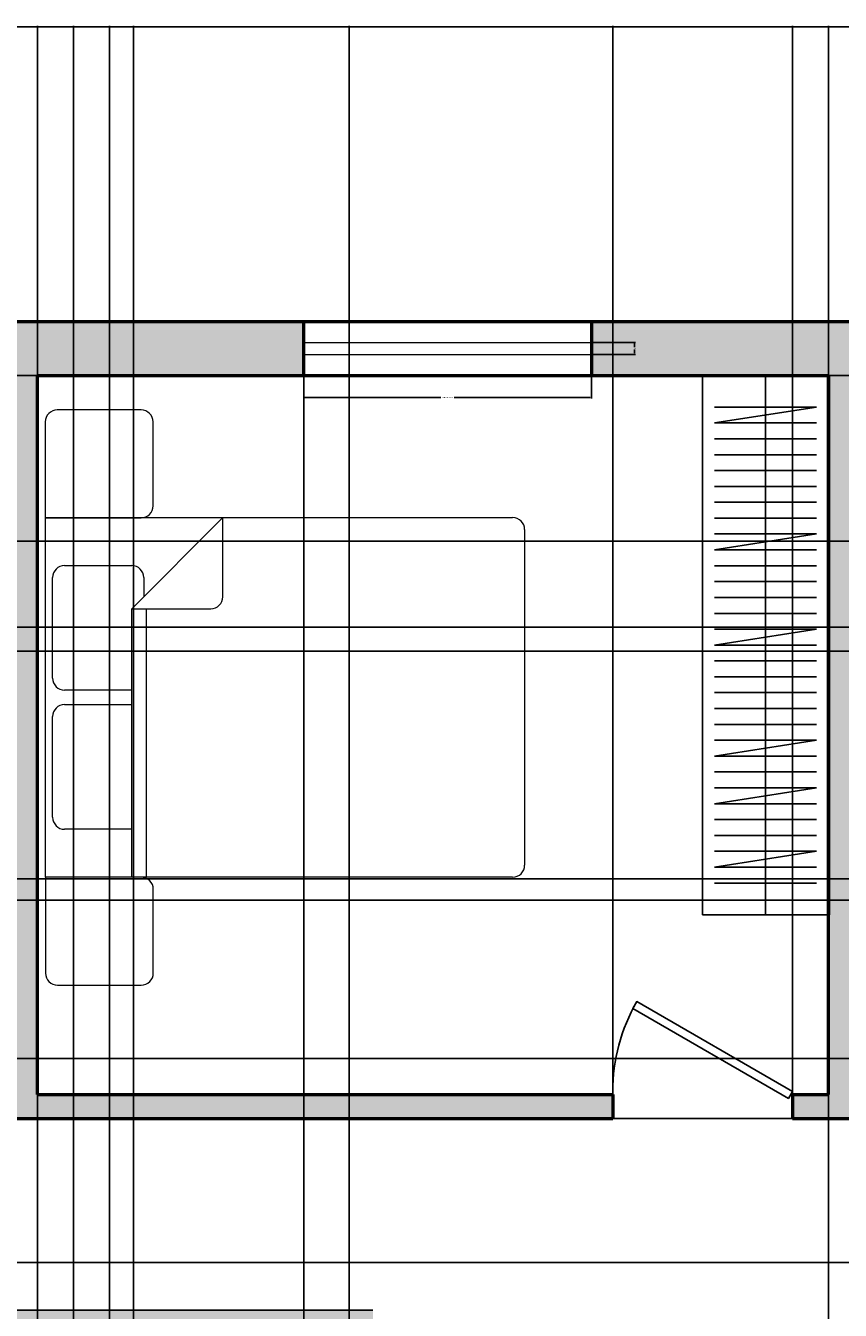
# Model space of a CAD drawing. Units: inches. Extents: x 1869 to 2483, y 2084 to 2479.
# Tile 4 of 7: x 1952 to 2088, y 2265 to 2479. Entities that reach past the tile are written whole.
import ezdxf

# ---------------------------------------------------------------- set-up
doc = ezdxf.new("R2010")
doc.units = ezdxf.units.IN
for name, color, linetype, lineweight in [('A-ANNO-DIMS', 2, 'Continuous', 18), ('A-DOOR', 3, 'Continuous', 25), ('A-FLOR-CASE', 9, 'Continuous', 25), ('A-FURN', 8, 'Continuous', 18), ('A-GLAZ', 4, 'Continuous', 18), ('A-WALL', 7, 'Continuous', 50)]:
    doc.layers.add(name, color=color, linetype=linetype, lineweight=lineweight)
doc.layers.add('A-WALL-PATT', color=18, linetype='Continuous', lineweight=13, true_color=0x000000)
doc.styles.get("Standard").update_dxf_attribs({"font": 'arial.ttf'})
doc.dimstyles.get("Standard").update_dxf_attribs({"dimtxt": 0.18, "dimasz": 0.18, "dimexe": 0.18, "dimexo": 0.0625, "dimgap": 0.09, "dimtad": 0, "dimtih": 1, "dimtoh": 1, "dimdec": 4, "dimzin": 0, "dimdsep": 46, "dimtxsty": 'Standard', "dimcen": 0.09, "dimadec": 0, "dimazin": 0, "dimtfac": 1, "dimtdec": 4, "dimtofl": 0, "dimtmove": 0, "dimatfit": 3, "dimfxl": 1, "dimtolj": 1, "dimtzin": 0, "dimarcsym": 0})

# ---------------------------------------------------------------- blocks, each defined once
blk = doc.blocks.new('Bed - Queen')
for p, q in [((0, -78), (0, 0)), ((0, 0), (60, 0)), ((60, 0), (60, -78)), ((10, -1.2), (26.8, -1.2)), ((33.2, -1.2), (50, -1.2)), ((8, -14.4), (8, -3.2)), ((28.8, -3.2), (28.8, -14.4)), ((31.2, -14.4), (31.2, -3.2)), ((52, -3.2), (52, -14.4)), ((0, -14.4), (44.8, -14.4)), ((60, -29.6), (44.8, -14.4)), ((44.8, -14.4), (44.8, -27.6)), ((44.8, -16.8), (0, -16.8)), ((50, -16.4), (46.8, -16.4)), ((46.8, -29.6), (60, -29.6)), ((58, -80), (2, -80))]:
    blk.add_line(p, q)
for points in [[(0, 0), (-16, 0, 0.414214), (-18, -2), (-18, -16, 0.414214), (-16, -18), (-2, -18, 0.414214), (0, -16)], [(75.96, 0.02), (59.96, 0.02), (59.96, -15.98, 0.414214), (61.96, -17.98), (75.96, -17.98, 0.414214), (77.96, -15.98), (77.96, -1.98, 0.414214)]]:
    blk.add_lwpolyline(points, format="xyb", close=True)
for centre, start, end in [((10, -3.2), 90, 180), ((26.8, -3.2), 0, 90), ((33.2, -3.2), 90, 180), ((50, -3.2), 0, 90), ((50, -14.4), 270, 0), ((46.8, -27.6), 180, 270), ((2, -78), 180, 270), ((58, -78), 270, 0)]:
    blk.add_arc(centre, 2, start, end)
blk = doc.blocks.new('*U12')
for p, q in [((0, 0), (0, -6)), ((-40, 0), (-40, -6))]:
    blk.add_line(p, q)
blk.add_lwpolyline([(0, 0), (-34.64, 20), (-35.52, 18.48), (-0.88, -1.52)], close=True)
blk.add_arc((0, 0), 40, 150, 180)
blk = doc.blocks.new('WIN-GLAZING-48IN')
for p, q in [((0, 2), (48, 2)), ((0, 0), (48, 0))]:
    blk.add_line(p, q)
blk = doc.blocks.new('WARDROBE-RAIL-90IN')
for p, q in [((8.5, 90), (8.5, 0)), ((0, 84.71), (17, 84.71)), ((17, 84.71), (0, 82.06)), ((0, 82.06), (17, 82.06)), ((0, 79.41), (17, 79.41)), ((0, 76.76), (17, 76.76)), ((0, 74.12), (17, 74.12)), ((0, 71.47), (17, 71.47)), ((0, 68.82), (17, 68.82)), ((0, 66.18), (17, 66.18)), ((0, 63.53), (17, 63.53)), ((17, 63.53), (0, 60.88)), ((0, 60.88), (17, 60.88)), ((0, 58.23), (17, 58.23)), ((0, 55.59), (17, 55.59)), ((0, 52.94), (17, 52.94)), ((0, 50.29), (17, 50.29)), ((0, 47.65), (17, 47.65)), ((17, 47.65), (0, 45)), ((0, 45), (17, 45)), ((0, 42.35), (17, 42.35)), ((0, 39.71), (17, 39.71)), ((0, 37.06), (17, 37.06)), ((0, 34.41), (17, 34.41)), ((0, 31.76), (17, 31.76)), ((0, 29.12), (17, 29.12)), ((17, 29.12), (0, 26.47)), ((0, 26.47), (17, 26.47)), ((0, 23.82), (17, 23.82)), ((0, 21.18), (17, 21.18)), ((17, 21.18), (0, 18.53)), ((0, 18.53), (17, 18.53)), ((0, 15.88), (17, 15.88)), ((0, 13.23), (17, 13.23)), ((0, 10.59), (17, 10.59)), ((17, 10.59), (0, 7.94)), ((0, 7.94), (17, 7.94)), ((0, 5.29), (17, 5.29))]:
    blk.add_line(p, q)
blk = doc.blocks.new('*D17')
at = {"layer": 'A-ANNO-DIMS', "color": 0, "lineweight": -2, "transparency": 16777216}
for p, q in [((1998.52, 2424.16), (1998.52, 2416.84)), ((2046.52, 2424.16), (2046.52, 2416.84)), ((1998.7, 2417.02), (2021.4, 2417.02)), ((2046.34, 2417.02), (2023.64, 2417.02))]:
    blk.add_line(p, q, dxfattribs=at)
at = {"layer": 'A-ANNO-DIMS', "color": 0, "transparency": 16777216}
for points in [[(1998.7, 2417.05), (1998.7, 2416.99), (1998.52, 2417.02)], [(2046.34, 2417.05), (2046.34, 2416.99), (2046.52, 2417.02)]]:
    blk.add_solid(points, dxfattribs=at)
at = {"layer": 'Defpoints', "color": 0, "transparency": 16777216}
for p in [(1998.52, 2424.22), (2046.52, 2424.22), (2046.52, 2417.02)]:
    blk.add_point(p, dxfattribs=at)
at = {"layer": 'A-ANNO-DIMS', "color": 0, "transparency": 16777216, "insert": (2022.52, 2417.02), "char_height": 0.18, "attachment_point": 5}
blk.add_mtext('\\A1;WINDOW 48 TYP.', dxfattribs=at)
blk = doc.blocks.new('*D18')
at = {"layer": 'A-ANNO-DIMS', "color": 0, "lineweight": -2, "transparency": 16777216}
for p, q in [((2046.58, 2426.22), (2053.9, 2426.22)), ((2053.72, 2426.04), (2053.72, 2425.4)), ((2053.72, 2424.4), (2053.72, 2425.04)), ((2046.58, 2424.22), (2053.9, 2424.22))]:
    blk.add_line(p, q, dxfattribs=at)
at = {"layer": 'A-ANNO-DIMS', "color": 0, "transparency": 16777216}
for points in [[(2053.69, 2426.04), (2053.75, 2426.04), (2053.72, 2426.22)], [(2053.69, 2424.4), (2053.75, 2424.4), (2053.72, 2424.22)]]:
    blk.add_solid(points, dxfattribs=at)
at = {"layer": 'Defpoints', "color": 0, "transparency": 16777216}
for p in [(2046.52, 2426.22), (2053.72, 2426.22), (2046.52, 2424.22)]:
    blk.add_point(p, dxfattribs=at)
at = {"layer": 'A-ANNO-DIMS', "color": 0, "transparency": 16777216, "insert": (2053.72, 2425.22), "char_height": 0.18, "attachment_point": 5}
blk.add_mtext('\\A1;2 TYP.', dxfattribs=at)
blk = doc.blocks.new('*D36')
at = {"layer": 'A-ANNO-DIMS', "color": 0, "lineweight": -2, "transparency": 16777216}
for p, q in [((1954.08, 2420.79), (1954.08, 2479.07)), ((1954.26, 2478.89), (2019.8, 2478.89)), ((2085.9, 2478.89), (2020.36, 2478.89)), ((2086.08, 2420.79), (2086.08, 2479.07))]:
    blk.add_line(p, q, dxfattribs=at)
at = {"layer": 'A-ANNO-DIMS', "color": 0, "transparency": 16777216}
for points in [[(1954.26, 2478.92), (1954.26, 2478.86), (1954.08, 2478.89)], [(2085.9, 2478.92), (2085.9, 2478.86), (2086.08, 2478.89)]]:
    blk.add_solid(points, dxfattribs=at)
at = {"layer": 'Defpoints', "color": 0, "transparency": 16777216}
for p in [(2086.08, 2478.89), (1954.08, 2420.72), (2086.08, 2420.72)]:
    blk.add_point(p, dxfattribs=at)
at = {"layer": 'A-ANNO-DIMS', "color": 0, "transparency": 16777216, "insert": (2020.08, 2478.89), "char_height": 0.18, "attachment_point": 5}
blk.add_mtext('\\A1;132', dxfattribs=at)
blk = doc.blocks.new('*D47')
at = {"layer": 'A-ANNO-DIMS', "color": 0, "lineweight": -2, "transparency": 16777216}
for p, q in [((2322.02, 2420.72), (1868.9, 2420.72)), ((1869.08, 2420.54), (1869.08, 2399.9)), ((1869.08, 2378.9), (1869.08, 2399.54)), ((2322.02, 2378.72), (1868.9, 2378.72))]:
    blk.add_line(p, q, dxfattribs=at)
at = {"layer": 'A-ANNO-DIMS', "color": 0, "transparency": 16777216}
for points in [[(1869.05, 2420.54), (1869.11, 2420.54), (1869.08, 2420.72)], [(1869.05, 2378.9), (1869.11, 2378.9), (1869.08, 2378.72)]]:
    blk.add_solid(points, dxfattribs=at)
at = {"layer": 'Defpoints', "color": 0, "transparency": 16777216}
for p in [(1869.08, 2420.72), (2322.08, 2420.72), (2322.08, 2378.72)]:
    blk.add_point(p, dxfattribs=at)
at = {"layer": 'A-ANNO-DIMS', "color": 0, "transparency": 16777216, "insert": (1869.08, 2399.72), "char_height": 0.18, "attachment_point": 5}
blk.add_mtext('\\A1;42', dxfattribs=at)
blk = doc.blocks.new('*D49')
at = {"layer": 'A-ANNO-DIMS', "color": 0, "lineweight": -2, "transparency": 16777216}
for p, q in [((1906.08, 2260.79), (1906.08, 2479.07)), ((1906.26, 2478.89), (1935.86, 2478.89)), ((1965.9, 2478.89), (1936.3, 2478.89)), ((1966.08, 2260.79), (1966.08, 2479.07))]:
    blk.add_line(p, q, dxfattribs=at)
at = {"layer": 'A-ANNO-DIMS', "color": 0, "transparency": 16777216}
for points in [[(1906.26, 2478.92), (1906.26, 2478.86), (1906.08, 2478.89)], [(1965.9, 2478.92), (1965.9, 2478.86), (1966.08, 2478.89)]]:
    blk.add_solid(points, dxfattribs=at)
at = {"layer": 'Defpoints', "color": 0, "transparency": 16777216}
for p in [(1966.08, 2478.89), (1906.08, 2260.72), (1966.08, 2260.72)]:
    blk.add_point(p, dxfattribs=at)
at = {"layer": 'A-ANNO-DIMS', "color": 0, "transparency": 16777216, "insert": (1936.08, 2478.89), "char_height": 0.18, "attachment_point": 5}
blk.add_mtext('\\A1;60', dxfattribs=at)
blk = doc.blocks.new('*D50')
at = {"layer": 'A-ANNO-DIMS', "color": 0, "lineweight": -2, "transparency": 16777216}
for p, q in [((1970.08, 2260.79), (1970.08, 2479.07)), ((1970.26, 2478.89), (1987.86, 2478.89)), ((2005.9, 2478.89), (1988.3, 2478.89)), ((2006.08, 2260.79), (2006.08, 2479.07))]:
    blk.add_line(p, q, dxfattribs=at)
at = {"layer": 'A-ANNO-DIMS', "color": 0, "transparency": 16777216}
for points in [[(1970.26, 2478.92), (1970.26, 2478.86), (1970.08, 2478.89)], [(2005.9, 2478.92), (2005.9, 2478.86), (2006.08, 2478.89)]]:
    blk.add_solid(points, dxfattribs=at)
at = {"layer": 'Defpoints', "color": 0, "transparency": 16777216}
for p in [(2006.08, 2478.89), (1970.08, 2260.72), (2006.08, 2260.72)]:
    blk.add_point(p, dxfattribs=at)
at = {"layer": 'A-ANNO-DIMS', "color": 0, "transparency": 16777216, "insert": (1988.08, 2478.89), "char_height": 0.18, "attachment_point": 5}
blk.add_mtext('\\A1;36', dxfattribs=at)
blk = doc.blocks.new('*D51')
at = {"layer": 'A-ANNO-DIMS', "color": 0, "lineweight": -2, "transparency": 16777216}
for p, q in [((1954.08, 2420.66), (1954.08, 2083.54)), ((1998.52, 2420.66), (1998.52, 2083.54)), ((1954.26, 2083.72), (1975.9, 2083.72)), ((1998.34, 2083.72), (1976.7, 2083.72))]:
    blk.add_line(p, q, dxfattribs=at)
at = {"layer": 'A-ANNO-DIMS', "color": 0, "transparency": 16777216}
for points in [[(1954.26, 2083.75), (1954.26, 2083.69), (1954.08, 2083.72)], [(1998.34, 2083.75), (1998.34, 2083.69), (1998.52, 2083.72)]]:
    blk.add_solid(points, dxfattribs=at)
at = {"layer": 'Defpoints', "color": 0, "transparency": 16777216}
for p in [(1954.08, 2420.72), (1998.52, 2420.72), (1998.52, 2083.72)]:
    blk.add_point(p, dxfattribs=at)
at = {"layer": 'A-ANNO-DIMS', "color": 0, "transparency": 16777216, "insert": (1976.3, 2083.72), "char_height": 0.18, "attachment_point": 5}
blk.add_mtext('\\A1;44.44', dxfattribs=at)
blk = doc.blocks.new('*D57')
at = {"layer": 'A-ANNO-DIMS', "color": 0, "lineweight": -2, "transparency": 16777216}
for p, q in [((2446.02, 2296.72), (1868.9, 2296.72)), ((1869.08, 2296.54), (1869.08, 2274.58)), ((1869.08, 2252.25), (1869.08, 2274.22)), ((2446.02, 2252.07), (1868.9, 2252.07))]:
    blk.add_line(p, q, dxfattribs=at)
at = {"layer": 'A-ANNO-DIMS', "color": 0, "transparency": 16777216}
for points in [[(1869.05, 2296.54), (1869.11, 2296.54), (1869.08, 2296.72)], [(1869.05, 2252.25), (1869.11, 2252.25), (1869.08, 2252.07)]]:
    blk.add_solid(points, dxfattribs=at)
at = {"layer": 'Defpoints', "color": 0, "transparency": 16777216}
for p in [(1869.08, 2296.72), (2446.08, 2296.72), (2446.08, 2252.07)]:
    blk.add_point(p, dxfattribs=at)
at = {"layer": 'A-ANNO-DIMS', "color": 0, "transparency": 16777216, "insert": (1869.08, 2274.4), "char_height": 0.18, "attachment_point": 5}
blk.add_mtext('\\A1;44.65', dxfattribs=at)
blk = doc.blocks.new('*D62')
at = {"layer": 'A-ANNO-DIMS', "color": 0, "lineweight": -2, "transparency": 16777216}
for p, q in [((2322.02, 2336.72), (1868.9, 2336.72)), ((1869.08, 2336.54), (1869.08, 2321.91)), ((1869.08, 2306.9), (1869.08, 2321.54)), ((2322.02, 2306.72), (1868.9, 2306.72))]:
    blk.add_line(p, q, dxfattribs=at)
at = {"layer": 'A-ANNO-DIMS', "color": 0, "transparency": 16777216}
for points in [[(1869.05, 2336.54), (1869.11, 2336.54), (1869.08, 2336.72)], [(1869.05, 2306.9), (1869.11, 2306.9), (1869.08, 2306.72)]]:
    blk.add_solid(points, dxfattribs=at)
at = {"layer": 'Defpoints', "color": 0, "transparency": 16777216}
for p in [(1869.08, 2336.72), (2322.08, 2336.72), (2322.08, 2306.72)]:
    blk.add_point(p, dxfattribs=at)
at = {"layer": 'A-ANNO-DIMS', "color": 0, "transparency": 16777216, "insert": (1869.08, 2321.72), "char_height": 0.18, "attachment_point": 5}
blk.add_mtext('\\A1;30', dxfattribs=at)
blk = doc.blocks.new('*D63')
at = {"layer": 'A-ANNO-DIMS', "color": 0, "lineweight": -2, "transparency": 16777216}
for p, q in [((2348.34, 2272.72), (1868.9, 2272.72)), ((1869.08, 2272.54), (1869.08, 2257.91)), ((1869.08, 2242.9), (1869.08, 2257.54)), ((2348.34, 2242.72), (1868.9, 2242.72))]:
    blk.add_line(p, q, dxfattribs=at)
at = {"layer": 'A-ANNO-DIMS', "color": 0, "transparency": 16777216}
for points in [[(1869.05, 2272.54), (1869.11, 2272.54), (1869.08, 2272.72)], [(1869.05, 2242.9), (1869.11, 2242.9), (1869.08, 2242.72)]]:
    blk.add_solid(points, dxfattribs=at)
at = {"layer": 'Defpoints', "color": 0, "transparency": 16777216}
for p in [(1869.08, 2272.72), (2348.4, 2272.72), (2348.4, 2242.72)]:
    blk.add_point(p, dxfattribs=at)
at = {"layer": 'A-ANNO-DIMS', "color": 0, "transparency": 16777216, "insert": (1869.08, 2257.72), "char_height": 0.18, "attachment_point": 5}
blk.add_mtext('\\A1;30', dxfattribs=at)
blk = doc.blocks.new('*D65')
at = {"layer": 'A-ANNO-DIMS', "color": 0, "lineweight": -2, "transparency": 16777216}
for p, q in [((2050.08, 2296.79), (2050.08, 2479.07)), ((2050.26, 2478.89), (2064.86, 2478.89)), ((2079.9, 2478.89), (2065.3, 2478.89)), ((2080.08, 2296.79), (2080.08, 2479.07))]:
    blk.add_line(p, q, dxfattribs=at)
at = {"layer": 'A-ANNO-DIMS', "color": 0, "transparency": 16777216}
for points in [[(2050.26, 2478.92), (2050.26, 2478.86), (2050.08, 2478.89)], [(2079.9, 2478.92), (2079.9, 2478.86), (2080.08, 2478.89)]]:
    blk.add_solid(points, dxfattribs=at)
at = {"layer": 'Defpoints', "color": 0, "transparency": 16777216}
for p in [(2080.08, 2478.89), (2050.08, 2296.72), (2080.08, 2296.72)]:
    blk.add_point(p, dxfattribs=at)
at = {"layer": 'A-ANNO-DIMS', "color": 0, "transparency": 16777216, "insert": (2065.08, 2478.89), "char_height": 0.18, "attachment_point": 5}
blk.add_mtext('\\A1;30', dxfattribs=at)
blk = doc.blocks.new('*D67')
at = {"layer": 'A-ANNO-DIMS', "color": 0, "lineweight": -2, "transparency": 16777216}
for p, q in [((1936.08, 2216.79), (1936.08, 2479.07)), ((1936.26, 2478.89), (1947.86, 2478.89)), ((1959.9, 2478.89), (1948.3, 2478.89)), ((1960.08, 2216.79), (1960.08, 2479.07))]:
    blk.add_line(p, q, dxfattribs=at)
at = {"layer": 'A-ANNO-DIMS', "color": 0, "transparency": 16777216}
for points in [[(1936.26, 2478.92), (1936.26, 2478.86), (1936.08, 2478.89)], [(1959.9, 2478.92), (1959.9, 2478.86), (1960.08, 2478.89)]]:
    blk.add_solid(points, dxfattribs=at)
at = {"layer": 'Defpoints', "color": 0, "transparency": 16777216}
for p in [(1960.08, 2478.89), (1936.08, 2216.72), (1960.08, 2216.72)]:
    blk.add_point(p, dxfattribs=at)
at = {"layer": 'A-ANNO-DIMS', "color": 0, "transparency": 16777216, "insert": (1948.08, 2478.89), "char_height": 0.18, "attachment_point": 5}
blk.add_mtext('\\A1;24', dxfattribs=at)
blk = doc.blocks.new('*D72')
at = {"layer": 'A-ANNO-DIMS', "color": 0, "lineweight": -2, "transparency": 16777216}
for p, q in [((2086.08, 2300.66), (2086.08, 2083.54)), ((2090.08, 2296.66), (2090.08, 2083.54)), ((2086.26, 2083.72), (2087.93, 2083.72)), ((2089.9, 2083.72), (2088.23, 2083.72))]:
    blk.add_line(p, q, dxfattribs=at)
at = {"layer": 'A-ANNO-DIMS', "color": 0, "transparency": 16777216}
for points in [[(2086.26, 2083.75), (2086.26, 2083.69), (2086.08, 2083.72)], [(2089.9, 2083.75), (2089.9, 2083.69), (2090.08, 2083.72)]]:
    blk.add_solid(points, dxfattribs=at)
at = {"layer": 'Defpoints', "color": 0, "transparency": 16777216}
for p in [(2086.08, 2300.72), (2090.08, 2296.72), (2090.08, 2083.72)]:
    blk.add_point(p, dxfattribs=at)
at = {"layer": 'A-ANNO-DIMS', "color": 0, "transparency": 16777216, "insert": (2088.08, 2083.72), "char_height": 0.18, "attachment_point": 5}
blk.add_mtext('\\A1;4', dxfattribs=at)
blk = doc.blocks.new('*D74')
at = {"layer": 'A-ANNO-DIMS', "color": 0, "lineweight": -2, "transparency": 16777216}
for p, q in [((1950.02, 2296.72), (1868.9, 2296.72)), ((1869.08, 2296.54), (1869.08, 2280.91)), ((1869.08, 2264.9), (1869.08, 2280.54)), ((2010.02, 2264.72), (1868.9, 2264.72))]:
    blk.add_line(p, q, dxfattribs=at)
at = {"layer": 'A-ANNO-DIMS', "color": 0, "transparency": 16777216}
for points in [[(1869.05, 2296.54), (1869.11, 2296.54), (1869.08, 2296.72)], [(1869.05, 2264.9), (1869.11, 2264.9), (1869.08, 2264.72)]]:
    blk.add_solid(points, dxfattribs=at)
at = {"layer": 'Defpoints', "color": 0, "transparency": 16777216}
for p in [(1869.08, 2296.72), (1950.08, 2296.72), (2010.08, 2264.72)]:
    blk.add_point(p, dxfattribs=at)
at = {"layer": 'A-ANNO-DIMS', "color": 0, "transparency": 16777216, "insert": (1869.08, 2280.72), "char_height": 0.18, "attachment_point": 5}
blk.add_mtext('\\A1;32', dxfattribs=at)
blk = doc.blocks.new('*D75')
at = {"layer": 'A-ANNO-DIMS', "color": 0, "lineweight": -2, "transparency": 16777216}
for p, q in [((1897.08, 2429.79), (1897.08, 2479.07)), ((1897.26, 2478.89), (2175.79, 2478.89)), ((2454.9, 2478.89), (2176.37, 2478.89)), ((2455.08, 2429.79), (2455.08, 2479.07))]:
    blk.add_line(p, q, dxfattribs=at)
at = {"layer": 'A-ANNO-DIMS', "color": 0, "transparency": 16777216}
for points in [[(1897.26, 2478.92), (1897.26, 2478.86), (1897.08, 2478.89)], [(2454.9, 2478.92), (2454.9, 2478.86), (2455.08, 2478.89)]]:
    blk.add_solid(points, dxfattribs=at)
at = {"layer": 'Defpoints', "color": 0, "transparency": 16777216}
for p in [(2455.08, 2478.89), (1897.08, 2429.72), (2455.08, 2429.72)]:
    blk.add_point(p, dxfattribs=at)
at = {"layer": 'A-ANNO-DIMS', "color": 0, "transparency": 16777216, "insert": (2176.08, 2478.89), "char_height": 0.18, "attachment_point": 5}
blk.add_mtext('\\A1;558', dxfattribs=at)
blk = doc.blocks.new('*D82')
at = {"layer": 'A-ANNO-DIMS', "color": 0, "lineweight": -2, "transparency": 16777216}
for p, q in [((2080.08, 2300.79), (2080.08, 2479.07)), ((2080.26, 2478.89), (2082.93, 2478.89)), ((2085.9, 2478.89), (2083.23, 2478.89)), ((2086.08, 2300.79), (2086.08, 2479.07))]:
    blk.add_line(p, q, dxfattribs=at)
at = {"layer": 'A-ANNO-DIMS', "color": 0, "transparency": 16777216}
for points in [[(2080.26, 2478.92), (2080.26, 2478.86), (2080.08, 2478.89)], [(2085.9, 2478.92), (2085.9, 2478.86), (2086.08, 2478.89)]]:
    blk.add_solid(points, dxfattribs=at)
at = {"layer": 'Defpoints', "color": 0, "transparency": 16777216}
for p in [(2086.08, 2478.89), (2080.08, 2300.72), (2086.08, 2300.72)]:
    blk.add_point(p, dxfattribs=at)
at = {"layer": 'A-ANNO-DIMS', "color": 0, "transparency": 16777216, "insert": (2083.08, 2478.89), "char_height": 0.18, "attachment_point": 5}
blk.add_mtext('\\A1;6', dxfattribs=at)
blk = doc.blocks.new('*D83')
at = {"layer": 'A-ANNO-DIMS', "color": 0, "lineweight": -2, "transparency": 16777216}
for p, q in [((1960.08, 2216.79), (1960.08, 2479.07)), ((1960.26, 2478.89), (1962.7, 2478.89)), ((1965.9, 2478.89), (1963.46, 2478.89)), ((1966.08, 2216.79), (1966.08, 2479.07))]:
    blk.add_line(p, q, dxfattribs=at)
at = {"layer": 'A-ANNO-DIMS', "color": 0, "transparency": 16777216}
for points in [[(1960.26, 2478.92), (1960.26, 2478.86), (1960.08, 2478.89)], [(1965.9, 2478.92), (1965.9, 2478.86), (1966.08, 2478.89)]]:
    blk.add_solid(points, dxfattribs=at)
at = {"layer": 'Defpoints', "color": 0, "transparency": 16777216}
for p in [(1966.08, 2478.89), (1960.08, 2216.72), (1966.08, 2216.72)]:
    blk.add_point(p, dxfattribs=at)
at = {"layer": 'A-ANNO-DIMS', "color": 0, "transparency": 16777216, "insert": (1963.08, 2478.89), "char_height": 0.18, "attachment_point": 5}
blk.add_mtext('\\A1;6.001', dxfattribs=at)
blk = doc.blocks.new('*D94')
at = {"layer": 'A-ANNO-DIMS', "color": 0, "lineweight": -2, "transparency": 16777216}
for p, q in [((2170.02, 2374.72), (1868.9, 2374.72)), ((1869.08, 2374.54), (1869.08, 2354.12)), ((1869.08, 2333.33), (1869.08, 2353.75)), ((2180.87, 2333.15), (1868.9, 2333.15))]:
    blk.add_line(p, q, dxfattribs=at)
at = {"layer": 'A-ANNO-DIMS', "color": 0, "transparency": 16777216}
for points in [[(1869.05, 2374.54), (1869.11, 2374.54), (1869.08, 2374.72)], [(1869.05, 2333.33), (1869.11, 2333.33), (1869.08, 2333.15)]]:
    blk.add_solid(points, dxfattribs=at)
at = {"layer": 'Defpoints', "color": 0, "transparency": 16777216}
for p in [(2170.08, 2374.72), (1869.08, 2333.15), (2180.94, 2333.15)]:
    blk.add_point(p, dxfattribs=at)
at = {"layer": 'A-ANNO-DIMS', "color": 0, "transparency": 16777216, "insert": (1869.08, 2353.94), "char_height": 0.18, "attachment_point": 5}
blk.add_mtext('\\A1;41.575', dxfattribs=at)
blk = doc.blocks.new('*D96')
at = {"layer": 'A-ANNO-DIMS', "color": 0, "lineweight": -2, "transparency": 16777216}
for p, q in [((2446.02, 2420.72), (1868.9, 2420.72)), ((1869.08, 2420.54), (1869.08, 2407.07)), ((1869.08, 2393.24), (1869.08, 2406.71)), ((2446.08, 2393.06), (1868.9, 2393.06))]:
    blk.add_line(p, q, dxfattribs=at)
at = {"layer": 'A-ANNO-DIMS', "color": 0, "transparency": 16777216}
for points in [[(1869.05, 2420.54), (1869.11, 2420.54), (1869.08, 2420.72)], [(1869.05, 2393.24), (1869.11, 2393.24), (1869.08, 2393.06)]]:
    blk.add_solid(points, dxfattribs=at)
at = {"layer": 'Defpoints', "color": 0, "transparency": 16777216}
for p in [(1869.08, 2420.72), (2446.08, 2420.72), (2446.14, 2393.06)]:
    blk.add_point(p, dxfattribs=at)
at = {"layer": 'A-ANNO-DIMS', "color": 0, "transparency": 16777216, "insert": (1869.08, 2406.89), "char_height": 0.18, "attachment_point": 5}
blk.add_mtext('\\A1;27.667', dxfattribs=at)

msp = doc.modelspace()

# ---------------------------------------------------------------- hatches: boundary and pattern name
at = {"layer": 'A-WALL-PATT'}
h = msp.add_hatch(color=256, dxfattribs=at)
h.dxf.hatch_style = 1
h.paths.add_polyline_path([(1998.5221, 2429.7235), (1897.0799, 2429.7235), (1897.0799, 2252.2488), (1906.0799, 2252.2488), (1906.0799, 2260.7235), (1966.0799, 2260.7235), (1966.0799, 2216.7235), (1960.0791, 2216.7235), (1960.0161, 2212.7235), (2050.0707, 2212.7235), (2050.1612, 2216.7235), (2010.0799, 2216.7235), (2010.0799, 2226.7235), (2006.0799, 2226.7235), (2006.0799, 2216.7235), (1970.0799, 2216.7235), (1970.0799, 2260.7235), (2006.0799, 2260.7235), (2006.0799, 2250.7235), (2010.0799, 2250.7235), (2010.0799, 2264.7235), (1906.0799, 2264.7235), (1906.0799, 2336.7235), (1920.0799, 2336.7235), (1920.0799, 2340.7235), (1906.0799, 2340.7235), (1906.0799, 2420.7235), (1950.0799, 2420.7235), (1950.0799, 2340.7235), (1944.0799, 2340.7235), (1944.0799, 2336.7235), (1950.0799, 2336.7235), (1950.0799, 2296.7235), (2050.0799, 2296.7235), (2050.0799, 2300.7235), (1954.0799, 2300.7235), (1954.0799, 2420.7235), (1998.5221, 2420.7235)])
h = msp.add_hatch(color=256, dxfattribs=at)
h.dxf.hatch_style = 1
h.paths.add_polyline_path([(2373.5248, 2429.7235), (2046.5221, 2429.7235), (2046.5221, 2420.7235), (2086.0799, 2420.7235), (2086.0799, 2330.7235), (2086.0799, 2300.7235), (2080.0799, 2300.7235), (2080.0799, 2296.7235), (2090.0799, 2296.7235), (2090.0799, 2374.7235), (2170.0799, 2374.7235), (2170.0799, 2378.7235), (2090.0799, 2378.7235), (2090.0799, 2420.7235), (2322.0799, 2420.7235), (2322.0799, 2378.7235), (2242.0799, 2378.7235), (2242.0799, 2374.7235), (2322.0799, 2374.7235), (2322.0799, 2336.7235), (2326.0799, 2336.7235), (2326.0799, 2420.7235), (2373.5248, 2420.7235)])

# ---------------------------------------------------------------- linework, layer by layer
at = {"layer": 'A-FLOR-CASE'}
for p, q in [((2065.0799, 2420.7235), (2086.0799, 2420.7235)), ((2065.0799, 2330.7235), (2065.0799, 2420.7235)), ((2086.0799, 2330.7235), (2065.0799, 2330.7235)), ((2065.0799, 2330.7235), (2086.0799, 2330.7235))]:
    msp.add_line(p, q, dxfattribs=at)
at = {"layer": 'A-WALL'}
for p, q in [((1998.5221, 2420.7235), (1998.5221, 2429.7235)), ((2046.5221, 2429.7235), (2046.5221, 2420.7235)), ((1954.0799, 2300.7235), (1954.0799, 2420.7235)), ((1954.0799, 2420.7235), (2086.0799, 2420.7235)), ((2086.0799, 2300.7235), (2086.0799, 2420.7235)), ((2086.0799, 2420.7235), (2086.0799, 2330.7235)), ((1954.0799, 2300.7235), (2050.0799, 2300.7235)), ((2050.0799, 2300.7235), (2050.0799, 2296.7235)), ((2080.0799, 2300.7235), (2080.0799, 2296.7235)), ((2080.0799, 2300.7235), (2086.0799, 2300.7235)), ((1950.0799, 2296.7235), (2050.0799, 2296.7235)), ((2080.0799, 2296.7235), (2090.0799, 2296.7235))]:
    msp.add_line(p, q, dxfattribs=at)
msp.add_lwpolyline([(2152.0799, 2111.7235), (1897.0799, 2111.7235), (1897.0799, 2429.7235), (2455.0799, 2429.7235), (2455.0799, 2111.7235), (2200.0799, 2111.7235)], dxfattribs=at)

# ---------------------------------------------------------------- block references
at = {"layer": 'A-DOOR', "xscale": 0.75, "yscale": 0.75, "zscale": 0.75}
msp.add_blockref('*U12', (2080.0799, 2301.2235), dxfattribs=at)
at = {"layer": 'A-FLOR-CASE'}
msp.add_blockref('WARDROBE-RAIL-90IN', (2067.08, 2330.724), dxfattribs=at)
at = {"layer": 'A-FURN', "rotation": 90}
msp.add_blockref('Bed - Queen', (1955.3786, 2336.9856), dxfattribs=at)
at = {"layer": 'A-GLAZ'}
msp.add_blockref('WIN-GLAZING-48IN', (1998.522, 2424.224), dxfattribs=at)

# ---------------------------------------------------------------- dimensions: what is measured, and where the dimension line sits
at = {"layer": 'A-ANNO-DIMS'}
for base, p1, p2, override, picture, middle in [((2455.0799, 2478.8871), (1897.0799, 2429.7235), (2455.0799, 2429.7235), {"dimdec": 0, "dimlfac": 1, "dimrnd": 0, "dimzin": 0, "dimdsep": 46, "dimlunit": 2}, '*D75', (2176.0799, 2478.8871)), ((1966.0799, 2478.8871), (1906.0799, 2260.7235), (1966.0799, 2260.7235), {"dimdec": 0, "dimlfac": 1, "dimrnd": 0, "dimzin": 0, "dimdsep": 46, "dimlunit": 2}, '*D49', (1936.0799, 2478.8871)), ((1960.0791, 2478.8871), (1936.0791, 2216.7235), (1960.0791, 2216.7235), {"dimdec": 0, "dimlfac": 1, "dimrnd": 0, "dimzin": 0, "dimdsep": 46, "dimlunit": 2}, '*D67', (1948.0791, 2478.8871)), ((2086.0799, 2478.8871), (1954.0799, 2420.7235), (2086.0799, 2420.7235), {"dimdec": 0, "dimlfac": 1, "dimrnd": 0, "dimzin": 0, "dimdsep": 46, "dimlunit": 2}, '*D36', (2020.0799, 2478.8871)), ((1966.0799, 2478.8871), (1960.0791, 2216.7235), (1966.0799, 2216.7235), {"dimdec": 3, "dimlfac": 1, "dimrnd": 0, "dimzin": 0, "dimdsep": 46, "dimlunit": 2}, '*D83', (1963.0795, 2478.8871)), ((2006.0799, 2478.8871), (1970.0799, 2260.7235), (2006.0799, 2260.7235), {"dimdec": 0, "dimlfac": 1, "dimrnd": 0, "dimzin": 0, "dimdsep": 46, "dimlunit": 2}, '*D50', (1988.0799, 2478.8871)), ((2080.0799, 2478.8871), (2050.0799, 2296.7235), (2080.0799, 2296.7235), {"dimdec": 0, "dimlfac": 1, "dimrnd": 0, "dimzin": 0, "dimdsep": 46, "dimlunit": 2}, '*D65', (2065.0799, 2478.8871)), ((2086.0799, 2478.8871), (2080.0799, 2300.7235), (2086.0799, 2300.7235), {"dimdec": 0, "dimlfac": 1, "dimrnd": 0, "dimzin": 0, "dimdsep": 46, "dimlunit": 2}, '*D82', (2083.0799, 2478.8871)), ((1998.5221, 2083.7235), (1954.0799, 2420.7235), (1998.5221, 2420.7235), {"dimdec": 2, "dimlfac": 1, "dimrnd": 0, "dimzin": 0, "dimdsep": 46, "dimlunit": 2}, '*D51', (1976.301, 2083.7235)), ((2090.0799, 2083.7235), (2086.0799, 2300.7235), (2090.0799, 2296.7235), {"dimdec": 0, "dimlfac": 1, "dimrnd": 0, "dimzin": 0, "dimdsep": 46, "dimlunit": 2}, '*D72', (2088.0799, 2083.7235))]:
    dim = msp.add_linear_dim(base=base, p1=p1, p2=p2, dimstyle='Standard', override=override, dxfattribs=at)
    dim.commit()
    dim.dimension.update_dxf_attribs({"geometry": picture, "text_midpoint": middle})
dim = msp.add_linear_dim(base=(2053.7221, 2426.2235), p1=(2046.5221, 2424.2235), p2=(2046.5221, 2426.2235), angle=90, text='<> TYP.', dimstyle='Standard', override={"dimdec": 0, "dimlfac": 1, "dimrnd": 0, "dimzin": 0, "dimdsep": 46, "dimlunit": 2}, dxfattribs=at)
dim.commit()
dim.dimension.update_dxf_attribs({"geometry": '*D18', "text_midpoint": (2053.7221, 2425.2235)})
dim = msp.add_linear_dim(base=(2046.5221, 2417.0235), p1=(1998.5221, 2424.2235), p2=(2046.5221, 2424.2235), text='WINDOW <> TYP.', dimstyle='Standard', override={"dimdec": 0, "dimlfac": 1, "dimrnd": 0, "dimzin": 0, "dimdsep": 46, "dimlunit": 2}, dxfattribs=at)
dim.commit()
dim.dimension.update_dxf_attribs({"geometry": '*D17', "text_midpoint": (2022.5221, 2417.0235)})
for base, p1, p2, override, picture, middle in [((1869.0799, 2420.7235), (2446.143, 2393.0569), (2446.0799, 2420.7235), {"dimdec": 3, "dimlfac": 1, "dimrnd": 0, "dimzin": 0, "dimdsep": 46, "dimlunit": 2}, '*D96', (1869.0799, 2406.8902)), ((1869.0799, 2420.7235), (2322.0799, 2378.7235), (2322.0799, 2420.7235), {"dimdec": 0, "dimlfac": 1, "dimrnd": 0, "dimzin": 0, "dimdsep": 46, "dimlunit": 2}, '*D47', (1869.0799, 2399.7235)), ((1869.0799, 2333.1488), (2170.0799, 2374.7235), (2180.9372, 2333.1488), {"dimdec": 3, "dimlfac": 1, "dimrnd": 0, "dimzin": 0, "dimdsep": 46, "dimlunit": 2}, '*D94', (1869.0799, 2353.9361)), ((1869.0799, 2336.7235), (2322.0799, 2306.7235), (2322.0799, 2336.7235), {"dimdec": 0, "dimlfac": 1, "dimrnd": 0, "dimzin": 0, "dimdsep": 46, "dimlunit": 2}, '*D62', (1869.0799, 2321.7235)), ((1869.0799, 2296.7235), (2446.0799, 2252.0706), (2446.0799, 2296.7235), {"dimdec": 2, "dimlfac": 1, "dimrnd": 0, "dimzin": 0, "dimdsep": 46, "dimlunit": 2}, '*D57', (1869.0799, 2274.3971)), ((1869.0799, 2296.7235), (2010.0799, 2264.7235), (1950.0799, 2296.7235), {"dimdec": 0, "dimlfac": 1, "dimrnd": 0, "dimzin": 0, "dimdsep": 46, "dimlunit": 2}, '*D74', (1869.0799, 2280.7235)), ((1869.0799, 2272.7235), (2348.3982, 2242.7235), (2348.3982, 2272.7235), {"dimdec": 0, "dimlfac": 1, "dimrnd": 0, "dimzin": 0, "dimdsep": 46, "dimlunit": 2}, '*D63', (1869.0799, 2257.7235))]:
    dim = msp.add_linear_dim(base=base, p1=p1, p2=p2, angle=90, dimstyle='Standard', override=override, dxfattribs=at)
    dim.commit()
    dim.dimension.update_dxf_attribs({"geometry": picture, "text_midpoint": middle})

doc.saveas('drawing.dxf')
